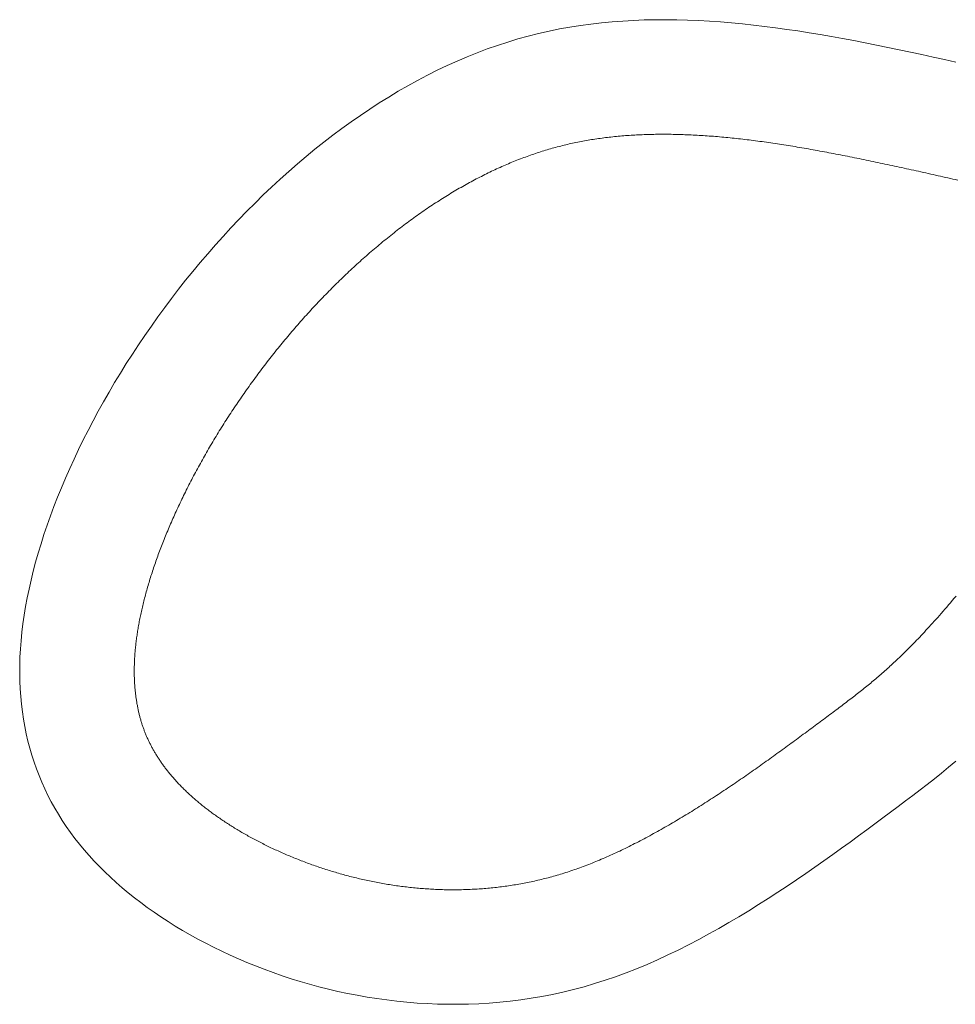
# Model space of a CAD drawing. Units: inches. Extents: x 64 to 1167, y 117 to 939.
# Tile 8 of 56: x 226.276 to 230.36, y 590.449 to 594.746. Entities that reach past the tile are written whole.
import ezdxf

# ---------------------------------------------------------------- set-up
doc = ezdxf.new("R2010")
doc.units = ezdxf.units.IN
doc.header["$MEASUREMENT"] = 0
doc.layers.add('A-FLOR-FIXT', color=8, linetype='Continuous', lineweight=18)

# ---------------------------------------------------------------- blocks, each defined once
blk = doc.blocks.new('FAUCET')
for points in [[(4.0816, 3.6354, 0), (4.1129, 3.6621, 0), (4.144, 3.6879, 0), (4.175, 3.713, 0), (4.2059, 3.7375, 0), (4.2371, 3.7616, 0), (4.2685, 3.7856, 0), (4.3004, 3.8096, 0), (4.3329, 3.8338, 0), (4.366, 3.8585, 0), (4.3999, 3.8837, 0), (4.4345, 3.9094, 0), (4.4699, 3.9356, 0), (4.506, 3.9621, 0), (4.5427, 3.989, 0), (4.5802, 4.0161, 0), (4.6182, 4.0434, 0), (4.6569, 4.0709, 0), (4.6961, 4.0984, 0), (4.7359, 4.126, 0), (4.7762, 4.1535, 0), (4.817, 4.181, 0), (4.8584, 4.2082, 0), (4.9002, 4.2353, 0), (4.9424, 4.2621, 0), (4.985, 4.2886, 0), (5.0281, 4.3147, 0), (5.0715, 4.3404, 0), (5.1152, 4.3655, 0), (5.1593, 4.3901, 0), (5.2036, 4.4141, 0), (5.2483, 4.4374, 0), (5.2931, 4.46, 0), (5.3382, 4.4817, 0), (5.3835, 4.5026, 0), (5.429, 4.5226, 0), (5.4746, 4.5416, 0), (5.5203, 4.5596, 0), (5.5662, 4.5765, 0), (5.6121, 4.5923, 0), (5.6581, 4.6068, 0), (5.7041, 4.6202, 0), (5.7502, 4.6325, 0), (5.7962, 4.6436, 0), (5.8423, 4.6537, 0), (5.8883, 4.6626, 0), (5.9343, 4.6705, 0), (5.9802, 4.6773, 0), (6.0261, 4.6831, 0), (6.0718, 4.6878, 0), (6.1175, 4.6916, 0), (6.163, 4.6944, 0), (6.2084, 4.6962, 0), (6.2536, 4.697, 0), (6.2986, 4.697, 0), (6.3435, 4.696, 0), (6.3882, 4.6942, 0), (6.4326, 4.6915, 0), (6.4768, 4.6879, 0), (6.5207, 4.6835, 0), (6.5644, 4.6782, 0), (6.6078, 4.6722, 0), (6.6509, 4.6654, 0), (6.6936, 4.6578, 0), (6.736, 4.6495, 0), (6.7781, 4.6405, 0), (6.8198, 4.6308, 0), (6.8611, 4.6203, 0), (6.902, 4.6092, 0), (6.9425, 4.5975, 0), (6.9825, 4.5851, 0), (7.0221, 4.5721, 0), (7.0612, 4.5585, 0), (7.0999, 4.5443, 0), (7.138, 4.5295, 0), (7.1756, 4.5143, 0), (7.2127, 4.4985, 0), (7.2492, 4.4821, 0), (7.2852, 4.4653, 0), (7.3206, 4.4481, 0), (7.3553, 4.4303, 0), (7.3895, 4.4122, 0), (7.423, 4.3936, 0), (7.4559, 4.3746, 0), (7.4881, 4.3553, 0), (7.5196, 4.3356, 0), (7.5504, 4.3155, 0), (7.5806, 4.2951, 0), (7.61, 4.2744, 0), (7.6387, 4.2533, 0), (7.6666, 4.2319, 0), (7.6939, 4.2101, 0), (7.7205, 4.188, 0), (7.7463, 4.1655, 0), (7.7714, 4.1426, 0), (7.7957, 4.1195, 0), (7.8193, 4.0959, 0), (7.8422, 4.072, 0), (7.8643, 4.0478, 0), (7.8857, 4.0231, 0), (7.9064, 3.9982, 0), (7.9262, 3.9728, 0), (7.9454, 3.9471, 0), (7.9637, 3.921, 0), (7.9813, 3.8946, 0), (7.9981, 3.8678, 0), (8.0142, 3.8406, 0), (8.0294, 3.8131, 0), (8.0439, 3.7852, 0), (8.0576, 3.7569, 0), (8.0705, 3.7282, 0), (8.0827, 3.6991, 0), (8.094, 3.6697, 0), (8.1045, 3.6399, 0), (8.1142, 3.6097, 0), (8.1231, 3.5791, 0), (8.1312, 3.5482, 0), (8.1385, 3.5168, 0), (8.145, 3.4851, 0), (8.1507, 3.453, 0), (8.1555, 3.4204, 0), (8.1595, 3.3875, 0), (8.1626, 3.3542, 0), (8.165, 3.3205, 0), (8.1665, 3.2864, 0), (8.1671, 3.252, 0), (8.1669, 3.2171, 0), (8.1659, 3.1818, 0), (8.164, 3.1461, 0), (8.1612, 3.11, 0), (8.1576, 3.0735, 0), (8.1531, 3.0366, 0), (8.1477, 2.9992, 0), (8.1415, 2.9615, 0), (8.1344, 2.9234, 0), (8.1264, 2.8849, 0), (8.1176, 2.846, 0), (8.108, 2.8068, 0), (8.0975, 2.7673, 0), (8.0862, 2.7275, 0), (8.074, 2.6874, 0), (8.0611, 2.647, 0), (8.0474, 2.6065, 0), (8.0329, 2.5657, 0), (8.0176, 2.5247, 0), (8.0016, 2.4835, 0), (7.9848, 2.4422, 0), (7.9672, 2.4008, 0), (7.9489, 2.3592, 0), (7.9299, 2.3176, 0), (7.9102, 2.2759, 0), (7.8898, 2.2341, 0), (7.8686, 2.1924, 0), (7.8468, 2.1506, 0), (7.8243, 2.1088, 0), (7.8011, 2.0671, 0), (7.7772, 2.0254, 0), (7.7527, 1.9838, 0), (7.7276, 1.9423, 0), (7.7018, 1.9009, 0), (7.6754, 1.8597, 0), (7.6484, 1.8186, 0), (7.6207, 1.7777, 0), (7.5925, 1.737, 0), (7.5637, 1.6965, 0), (7.5343, 1.6563, 0), (7.5043, 1.6163, 0), (7.4738, 1.5766, 0), (7.4428, 1.5372, 0), (7.4112, 1.4981, 0), (7.379, 1.4594, 0), (7.3464, 1.4211, 0), (7.3132, 1.3831, 0), (7.2795, 1.3456, 0), (7.2453, 1.3085, 0), (7.2107, 1.2718, 0), (7.1755, 1.2356, 0), (7.1399, 1.1999, 0), (7.1039, 1.1647, 0), (7.0674, 1.13, 0), (7.0305, 1.0959, 0), (6.9931, 1.0624, 0), (6.9553, 1.0294, 0), (6.9171, 0.9971, 0), (6.8785, 0.9654, 0), (6.8396, 0.9344, 0), (6.8002, 0.904, 0), (6.7605, 0.8744, 0), (6.7204, 0.8455, 0), (6.6799, 0.8173, 0), (6.6391, 0.7898, 0), (6.598, 0.7632, 0), (6.5566, 0.7373, 0), (6.5148, 0.7123, 0), (6.4727, 0.6881, 0), (6.4304, 0.6648, 0), (6.3877, 0.6424, 0), (6.3448, 0.6208, 0), (6.3016, 0.6002, 0), (6.2581, 0.5806, 0), (6.2144, 0.5619, 0), (6.1705, 0.5442, 0), (6.1263, 0.5275, 0), (6.0819, 0.5119, 0), (6.0373, 0.4973, 0), (5.9925, 0.4837, 0), (5.9475, 0.4713, 0), (5.9023, 0.4599, 0), (5.8569, 0.4497, 0), (5.8114, 0.4404, 0), (5.7657, 0.4322, 0), (5.7198, 0.425, 0), (5.6737, 0.4187, 0), (5.6275, 0.4134, 0), (5.5811, 0.409, 0), (5.5345, 0.4055, 0), (5.4878, 0.4029, 0), (5.441, 0.401, 0), (5.394, 0.4, 0), (5.3468, 0.3998, 0), (5.2995, 0.4004, 0), (5.2521, 0.4017, 0), (5.2045, 0.4036, 0), (5.1568, 0.4063, 0), (5.109, 0.4096, 0), (5.0611, 0.4136, 0), (5.013, 0.4182, 0), (4.9648, 0.4233, 0), (4.9165, 0.429, 0), (4.8681, 0.4352, 0), (4.8196, 0.4419, 0), (4.771, 0.4491, 0), (4.7222, 0.4568, 0), (4.6734, 0.4648, 0), (4.6245, 0.4733, 0), (4.5755, 0.4822, 0), (4.5264, 0.4913, 0), (4.4772, 0.5008, 0), (4.428, 0.5106, 0), (4.3786, 0.5207, 0), (4.3292, 0.531, 0), (4.2798, 0.5415, 0), (4.2302, 0.5522, 0), (4.1806, 0.5631, 0), (4.131, 0.5741, 0), (4.0812, 0.5853, 0)], [(4.0798, 2.9151, 0), (4.0883, 2.9251, 0), (4.0967, 2.935, 0), (4.1049, 2.9447, 0), (4.1131, 2.9542, 0), (4.1212, 2.9636, 0), (4.1292, 2.9729, 0), (4.1371, 2.9819, 0), (4.145, 2.9909, 0), (4.1527, 2.9996, 0), (4.1603, 3.0083, 0), (4.1679, 3.0168, 0), (4.1754, 3.0251, 0), (4.1828, 3.0333, 0), (4.1901, 3.0414, 0), (4.1973, 3.0493, 0), (4.2045, 3.0572, 0), (4.2116, 3.0648, 0), (4.2186, 3.0724, 0), (4.2256, 3.0798, 0), (4.2324, 3.0871, 0), (4.2392, 3.0943, 0), (4.246, 3.1013, 0), (4.2526, 3.1083, 0), (4.2592, 3.1151, 0), (4.2658, 3.1219, 0), (4.2722, 3.1285, 0), (4.2786, 3.135, 0), (4.285, 3.1414, 0), (4.2913, 3.1477, 0), (4.2975, 3.1539, 0), (4.3037, 3.16, 0), (4.3098, 3.166, 0), (4.3159, 3.1719, 0), (4.3219, 3.1777, 0), (4.3279, 3.1835, 0), (4.3338, 3.1891, 0), (4.3397, 3.1947, 0), (4.3456, 3.2002, 0), (4.3514, 3.2057, 0), (4.3572, 3.211, 0), (4.3629, 3.2164, 0), (4.3687, 3.2216, 0), (4.3744, 3.2268, 0), (4.3801, 3.2319, 0), (4.3857, 3.237, 0), (4.3914, 3.242, 0), (4.397, 3.247, 0), (4.4026, 3.252, 0), (4.4082, 3.2569, 0), (4.4138, 3.2617, 0), (4.4194, 3.2665, 0), (4.425, 3.2713, 0), (4.4306, 3.2761, 0), (4.4362, 3.2808, 0), (4.4418, 3.2855, 0), (4.4474, 3.2902, 0), (4.453, 3.2948, 0), (4.4587, 3.2995, 0), (4.4643, 3.3041, 0), (4.47, 3.3087, 0), (4.4756, 3.3133, 0), (4.4813, 3.3179, 0), (4.4871, 3.3224, 0), (4.4928, 3.327, 0), (4.4986, 3.3316, 0), (4.5044, 3.3362, 0), (4.5103, 3.3408, 0), (4.5161, 3.3454, 0), (4.5221, 3.35, 0), (4.528, 3.3546, 0), (4.534, 3.3592, 0), (4.5401, 3.3639, 0), (4.5462, 3.3685, 0), (4.5523, 3.3732, 0), (4.5585, 3.378, 0), (4.5648, 3.3827, 0), (4.5711, 3.3875, 0), (4.5775, 3.3923, 0), (4.5839, 3.3972, 0), (4.5905, 3.4021, 0), (4.597, 3.407, 0), (4.6037, 3.412, 0), (4.6104, 3.417, 0), (4.6172, 3.4221, 0), (4.624, 3.4272, 0), (4.6309, 3.4324, 0), (4.6379, 3.4376, 0), (4.6448, 3.4428, 0), (4.6519, 3.448, 0), (4.659, 3.4533, 0), (4.6661, 3.4586, 0), (4.6733, 3.464, 0), (4.6805, 3.4694, 0), (4.6877, 3.4748, 0), (4.695, 3.4802, 0), (4.7024, 3.4856, 0), (4.7097, 3.4911, 0), (4.7171, 3.4966, 0), (4.7246, 3.5021, 0), (4.732, 3.5076, 0), (4.7395, 3.5132, 0), (4.747, 3.5187, 0), (4.7546, 3.5243, 0), (4.7621, 3.5299, 0), (4.7697, 3.5355, 0), (4.7773, 3.541, 0), (4.7849, 3.5466, 0), (4.7926, 3.5523, 0), (4.8002, 3.5579, 0), (4.8079, 3.5635, 0), (4.8156, 3.5691, 0), (4.8232, 3.5747, 0), (4.8309, 3.5803, 0), (4.8386, 3.5859, 0), (4.8464, 3.5915, 0), (4.8541, 3.5972, 0), (4.8619, 3.6028, 0), (4.8696, 3.6084, 0), (4.8774, 3.614, 0), (4.8852, 3.6196, 0), (4.8931, 3.6253, 0), (4.9009, 3.6309, 0), (4.9088, 3.6365, 0), (4.9167, 3.6421, 0), (4.9246, 3.6478, 0), (4.9325, 3.6534, 0), (4.9404, 3.659, 0), (4.9484, 3.6646, 0), (4.9563, 3.6702, 0), (4.9643, 3.6758, 0), (4.9723, 3.6814, 0), (4.9803, 3.687, 0), (4.9883, 3.6926, 0), (4.9964, 3.6982, 0), (5.0044, 3.7038, 0), (5.0125, 3.7094, 0), (5.0206, 3.7149, 0), (5.0286, 3.7205, 0), (5.0367, 3.726, 0), (5.0449, 3.7316, 0), (5.053, 3.7371, 0), (5.0611, 3.7426, 0), (5.0693, 3.7481, 0), (5.0774, 3.7536, 0), (5.0856, 3.7591, 0), (5.0938, 3.7645, 0), (5.102, 3.77, 0), (5.1102, 3.7754, 0), (5.1184, 3.7808, 0), (5.1266, 3.7862, 0), (5.1349, 3.7916, 0), (5.1431, 3.797, 0), (5.1514, 3.8023, 0), (5.1596, 3.8077, 0), (5.1679, 3.813, 0), (5.1762, 3.8183, 0), (5.1844, 3.8235, 0), (5.1927, 3.8288, 0), (5.201, 3.834, 0), (5.2093, 3.8393, 0), (5.2176, 3.8444, 0), (5.2259, 3.8496, 0), (5.2342, 3.8548, 0), (5.2425, 3.8599, 0), (5.2509, 3.865, 0), (5.2592, 3.8701, 0), (5.2675, 3.8751, 0), (5.2758, 3.8801, 0), (5.2841, 3.8851, 0), (5.2925, 3.8901, 0), (5.3008, 3.8951, 0), (5.3091, 3.9, 0), (5.3174, 3.9049, 0), (5.3258, 3.9097, 0), (5.3341, 3.9146, 0), (5.3424, 3.9194, 0), (5.3507, 3.9241, 0), (5.359, 3.9289, 0), (5.3673, 3.9336, 0), (5.3757, 3.9382, 0), (5.384, 3.9429, 0), (5.3923, 3.9475, 0), (5.4005, 3.9521, 0), (5.4088, 3.9566, 0), (5.4171, 3.9611, 0), (5.4254, 3.9656, 0), (5.4337, 3.97, 0), (5.4419, 3.9744, 0), (5.4502, 3.9788, 0), (5.4584, 3.9831, 0), (5.4667, 3.9874, 0), (5.4749, 3.9916, 0), (5.4831, 3.9959, 0), (5.4913, 4, 0), (5.4995, 4.0042, 0), (5.5077, 4.0082, 0), (5.5159, 4.0123, 0), (5.5241, 4.0163, 0), (5.5322, 4.0203, 0), (5.5403, 4.0242, 0), (5.5485, 4.028, 0), (5.5566, 4.0319, 0), (5.5647, 4.0357, 0), (5.5728, 4.0394, 0), (5.5808, 4.0431, 0), (5.5889, 4.0467, 0), (5.5969, 4.0503, 0), (5.6049, 4.0539, 0), (5.6129, 4.0574, 0), (5.6209, 4.0608, 0), (5.6288, 4.0642, 0), (5.6367, 4.0676, 0), (5.6446, 4.0708, 0), (5.6525, 4.0741, 0), (5.6604, 4.0773, 0), (5.6682, 4.0804, 0), (5.676, 4.0835, 0), (5.6838, 4.0866, 0), (5.6916, 4.0896, 0), (5.6994, 4.0926, 0), (5.7072, 4.0955, 0), (5.7149, 4.0983, 0), (5.7226, 4.1012, 0), (5.7304, 4.1039, 0), (5.7381, 4.1067, 0), (5.7457, 4.1093, 0), (5.7534, 4.112, 0), (5.7611, 4.1146, 0), (5.7687, 4.1171, 0), (5.7764, 4.1196, 0), (5.784, 4.1221, 0), (5.7916, 4.1245, 0), (5.7992, 4.1269, 0), (5.8069, 4.1292, 0), (5.8144, 4.1315, 0), (5.822, 4.1337, 0), (5.8296, 4.1359, 0), (5.8372, 4.1381, 0), (5.8448, 4.1402, 0), (5.8523, 4.1422, 0), (5.8599, 4.1443, 0), (5.8674, 4.1462, 0), (5.875, 4.1482, 0), (5.8825, 4.1501, 0), (5.89, 4.1519, 0), (5.8976, 4.1538, 0), (5.9051, 4.1555, 0), (5.9126, 4.1573, 0), (5.9202, 4.159, 0), (5.9277, 4.1606, 0), (5.9352, 4.1623, 0), (5.9428, 4.1638, 0), (5.9503, 4.1654, 0), (5.9578, 4.1669, 0), (5.9654, 4.1683, 0), (5.9729, 4.1698, 0), (5.9804, 4.1712, 0), (5.988, 4.1725, 0), (5.9955, 4.1738, 0), (6.0031, 4.1751, 0), (6.0106, 4.1763, 0), (6.0182, 4.1775, 0), (6.0257, 4.1787, 0), (6.0333, 4.1798, 0), (6.0409, 4.1809, 0), (6.0485, 4.182, 0), (6.056, 4.183, 0), (6.0636, 4.184, 0), (6.0712, 4.1849, 0), (6.0788, 4.1858, 0), (6.0864, 4.1867, 0), (6.094, 4.1875, 0), (6.1016, 4.1883, 0), (6.1092, 4.1891, 0), (6.1168, 4.1898, 0), (6.1244, 4.1905, 0), (6.132, 4.1912, 0), (6.1396, 4.1918, 0), (6.1472, 4.1924, 0), (6.1548, 4.193, 0), (6.1624, 4.1935, 0), (6.17, 4.194, 0), (6.1776, 4.1944, 0), (6.1852, 4.1948, 0), (6.1928, 4.1952, 0), (6.2004, 4.1956, 0), (6.208, 4.1959, 0), (6.2155, 4.1961, 0), (6.2231, 4.1964, 0), (6.2307, 4.1966, 0), (6.2383, 4.1968, 0), (6.2459, 4.1969, 0), (6.2534, 4.197, 0), (6.261, 4.1971, 0), (6.2686, 4.1971, 0), (6.2761, 4.1971, 0), (6.2837, 4.1971, 0), (6.2913, 4.197, 0), (6.2988, 4.1969, 0), (6.3064, 4.1968, 0), (6.3139, 4.1967, 0), (6.3215, 4.1965, 0), (6.329, 4.1962, 0), (6.3365, 4.196, 0), (6.3441, 4.1957, 0), (6.3516, 4.1954, 0), (6.3591, 4.195, 0), (6.3666, 4.1946, 0), (6.3741, 4.1942, 0), (6.3817, 4.1937, 0), (6.3892, 4.1933, 0), (6.3967, 4.1927, 0), (6.4042, 4.1922, 0), (6.4116, 4.1916, 0), (6.4191, 4.191, 0), (6.4266, 4.1904, 0), (6.4341, 4.1897, 0), (6.4415, 4.189, 0), (6.449, 4.1883, 0), (6.4564, 4.1875, 0), (6.4639, 4.1867, 0), (6.4713, 4.1859, 0), (6.4788, 4.185, 0), (6.4862, 4.1841, 0), (6.4936, 4.1832, 0), (6.501, 4.1823, 0), (6.5084, 4.1813, 0), (6.5158, 4.1803, 0), (6.5232, 4.1793, 0), (6.5306, 4.1782, 0), (6.5379, 4.1771, 0), (6.5453, 4.176, 0), (6.5527, 4.1748, 0), (6.56, 4.1736, 0), (6.5673, 4.1724, 0), (6.5747, 4.1712, 0), (6.582, 4.1699, 0), (6.5893, 4.1686, 0), (6.5966, 4.1673, 0), (6.6039, 4.1659, 0), (6.6112, 4.1645, 0), (6.6185, 4.1631, 0), (6.6257, 4.1616, 0), (6.633, 4.1602, 0), (6.6402, 4.1587, 0), (6.6474, 4.1571, 0), (6.6546, 4.1556, 0), (6.6618, 4.154, 0), (6.669, 4.1524, 0), (6.6762, 4.1507, 0), (6.6834, 4.1491, 0), (6.6905, 4.1474, 0), (6.6977, 4.1457, 0), (6.7048, 4.1439, 0), (6.7119, 4.1421, 0), (6.719, 4.1403, 0), (6.7261, 4.1385, 0), (6.7332, 4.1367, 0), (6.7403, 4.1348, 0), (6.7473, 4.1329, 0), (6.7543, 4.131, 0), (6.7613, 4.129, 0), (6.7683, 4.1271, 0), (6.7753, 4.1251, 0), (6.7823, 4.123, 0), (6.7893, 4.121, 0), (6.7962, 4.1189, 0), (6.8031, 4.1168, 0), (6.81, 4.1147, 0), (6.8169, 4.1126, 0), (6.8238, 4.1104, 0), (6.8307, 4.1082, 0), (6.8375, 4.106, 0), (6.8443, 4.1038, 0), (6.8511, 4.1016, 0), (6.8579, 4.0993, 0), (6.8647, 4.097, 0), (6.8714, 4.0947, 0), (6.8782, 4.0924, 0), (6.8849, 4.09, 0), (6.8916, 4.0876, 0), (6.8982, 4.0852, 0), (6.9049, 4.0828, 0), (6.9115, 4.0804, 0), (6.9181, 4.0779, 0), (6.9247, 4.0754, 0), (6.9313, 4.0729, 0), (6.9379, 4.0704, 0), (6.9444, 4.0679, 0), (6.9509, 4.0653, 0), (6.9574, 4.0628, 0), (6.9639, 4.0602, 0), (6.9703, 4.0576, 0), (6.9767, 4.0549, 0), (6.9831, 4.0523, 0), (6.9895, 4.0496, 0), (6.9959, 4.047, 0), (7.0022, 4.0443, 0), (7.0085, 4.0415, 0), (7.0148, 4.0388, 0), (7.0211, 4.0361, 0), (7.0273, 4.0333, 0), (7.0335, 4.0305, 0), (7.0397, 4.0277, 0), (7.0459, 4.0249, 0), (7.052, 4.0221, 0), (7.0582, 4.0192, 0), (7.0642, 4.0164, 0), (7.0703, 4.0135, 0), (7.0764, 4.0106, 0), (7.0824, 4.0077, 0), (7.0884, 4.0048, 0), (7.0943, 4.0018, 0), (7.1003, 3.9989, 0), (7.1062, 3.9959, 0), (7.1121, 3.9929, 0), (7.1179, 3.99, 0), (7.1238, 3.987, 0), (7.1296, 3.9839, 0), (7.1353, 3.9809, 0), (7.1411, 3.9779, 0), (7.1468, 3.9748, 0), (7.1525, 3.9717, 0), (7.1582, 3.9687, 0), (7.1638, 3.9656, 0), (7.1694, 3.9625, 0), (7.175, 3.9593, 0), (7.1805, 3.9562, 0), (7.186, 3.9531, 0), (7.1915, 3.9499, 0), (7.197, 3.9468, 0), (7.2024, 3.9436, 0), (7.2078, 3.9404, 0), (7.2131, 3.9372, 0), (7.2185, 3.934, 0), (7.2238, 3.9308, 0), (7.229, 3.9276, 0), (7.2343, 3.9244, 0), (7.2395, 3.9211, 0), (7.2447, 3.9179, 0), (7.2498, 3.9146, 0), (7.2549, 3.9114, 0), (7.26, 3.9081, 0), (7.265, 3.9048, 0), (7.27, 3.9015, 0), (7.2749, 3.8983, 0), (7.2798, 3.895, 0), (7.2847, 3.8917, 0), (7.2895, 3.8884, 0), (7.2943, 3.8851, 0), (7.2991, 3.8819, 0), (7.3038, 3.8786, 0), (7.3085, 3.8753, 0), (7.3131, 3.872, 0), (7.3177, 3.8687, 0), (7.3223, 3.8654, 0), (7.3268, 3.8621, 0), (7.3313, 3.8588, 0), (7.3357, 3.8555, 0), (7.3401, 3.8522, 0), (7.3445, 3.8489, 0), (7.3488, 3.8456, 0), (7.3531, 3.8423, 0), (7.3574, 3.839, 0), (7.3616, 3.8357, 0), (7.3658, 3.8324, 0), (7.37, 3.8291, 0), (7.3741, 3.8258, 0), (7.3782, 3.8224, 0), (7.3822, 3.8191, 0), (7.3862, 3.8158, 0), (7.3902, 3.8125, 0), (7.3941, 3.8092, 0), (7.398, 3.8059, 0), (7.4019, 3.8025, 0), (7.4057, 3.7992, 0), (7.4095, 3.7959, 0), (7.4133, 3.7926, 0), (7.417, 3.7892, 0), (7.4207, 3.7859, 0), (7.4243, 3.7826, 0), (7.4279, 3.7793, 0), (7.4315, 3.7759, 0), (7.4351, 3.7726, 0), (7.4386, 3.7693, 0), (7.4421, 3.7659, 0), (7.4455, 3.7626, 0), (7.4489, 3.7593, 0), (7.4523, 3.7559, 0), (7.4557, 3.7526, 0), (7.459, 3.7493, 0), (7.4623, 3.7459, 0), (7.4655, 3.7426, 0), (7.4687, 3.7393, 0), (7.4719, 3.7359, 0), (7.4751, 3.7326, 0), (7.4782, 3.7293, 0), (7.4813, 3.7259, 0), (7.4843, 3.7226, 0), (7.4874, 3.7193, 0), (7.4903, 3.7159, 0), (7.4933, 3.7126, 0), (7.4962, 3.7093, 0), (7.4991, 3.7059, 0), (7.502, 3.7026, 0), (7.5048, 3.6992, 0), (7.5076, 3.6959, 0), (7.5104, 3.6926, 0), (7.5132, 3.6892, 0), (7.5159, 3.6859, 0), (7.5185, 3.6826, 0), (7.5212, 3.6792, 0), (7.5238, 3.6759, 0), (7.5264, 3.6726, 0), (7.529, 3.6692, 0), (7.5315, 3.6659, 0), (7.534, 3.6626, 0), (7.5365, 3.6592, 0), (7.5389, 3.6559, 0), (7.5413, 3.6526, 0), (7.5437, 3.6492, 0), (7.5461, 3.6459, 0), (7.5484, 3.6426, 0), (7.5507, 3.6392, 0), (7.553, 3.6359, 0), (7.5552, 3.6326, 0), (7.5574, 3.6293, 0), (7.5597, 3.6259, 0), (7.5618, 3.6226, 0), (7.564, 3.6193, 0), (7.5661, 3.6159, 0), (7.5682, 3.6126, 0), (7.5703, 3.6092, 0), (7.5724, 3.6059, 0), (7.5744, 3.6026, 0), (7.5764, 3.5992, 0), (7.5784, 3.5959, 0), (7.5803, 3.5925, 0), (7.5823, 3.5891, 0), (7.5842, 3.5858, 0), (7.5861, 3.5824, 0), (7.5879, 3.579, 0), (7.5898, 3.5757, 0), (7.5916, 3.5723, 0), (7.5934, 3.5689, 0), (7.5952, 3.5655, 0), (7.5969, 3.5621, 0), (7.5987, 3.5587, 0), (7.6004, 3.5553, 0), (7.602, 3.5518, 0), (7.6037, 3.5484, 0), (7.6053, 3.545, 0), (7.6069, 3.5415, 0), (7.6085, 3.538, 0), (7.6101, 3.5346, 0), (7.6116, 3.5311, 0), (7.6132, 3.5276, 0), (7.6147, 3.5241, 0), (7.6161, 3.5206, 0), (7.6176, 3.5171, 0), (7.619, 3.5136, 0), (7.6204, 3.51, 0), (7.6218, 3.5065, 0), (7.6232, 3.5029, 0), (7.6245, 3.4994, 0), (7.6259, 3.4958, 0), (7.6272, 3.4922, 0), (7.6284, 3.4886, 0), (7.6297, 3.4849, 0), (7.6309, 3.4813, 0), (7.6322, 3.4777, 0), (7.6333, 3.474, 0), (7.6345, 3.4703, 0), (7.6357, 3.4666, 0), (7.6368, 3.4629, 0), (7.6379, 3.4592, 0), (7.639, 3.4555, 0), (7.6401, 3.4517, 0), (7.6411, 3.4479, 0), (7.6421, 3.4441, 0), (7.6432, 3.4403, 0), (7.6441, 3.4365, 0), (7.6451, 3.4327, 0), (7.646, 3.4288, 0), (7.647, 3.4249, 0), (7.6479, 3.4211, 0), (7.6488, 3.4171, 0), (7.6496, 3.4132, 0), (7.6505, 3.4093, 0), (7.6513, 3.4053, 0), (7.6521, 3.4013, 0), (7.6529, 3.3973, 0), (7.6536, 3.3933, 0), (7.6544, 3.3892, 0), (7.6551, 3.3852, 0), (7.6558, 3.3811, 0), (7.6565, 3.377, 0), (7.6572, 3.3728, 0), (7.6578, 3.3687, 0), (7.6584, 3.3645, 0), (7.6591, 3.3603, 0), (7.6596, 3.3561, 0), (7.6602, 3.3518, 0), (7.6608, 3.3475, 0), (7.6613, 3.3432, 0), (7.6618, 3.3389, 0), (7.6623, 3.3346, 0), (7.6628, 3.3302, 0), (7.6632, 3.3258, 0), (7.6636, 3.3213, 0), (7.664, 3.3169, 0), (7.6644, 3.3124, 0), (7.6647, 3.3079, 0), (7.6651, 3.3033, 0), (7.6654, 3.2988, 0), (7.6657, 3.2941, 0), (7.6659, 3.2895, 0), (7.6661, 3.2849, 0), (7.6663, 3.2802, 0), (7.6665, 3.2755, 0), (7.6667, 3.2707, 0), (7.6668, 3.2659, 0), (7.6669, 3.2611, 0), (7.667, 3.2563, 0), (7.6671, 3.2514, 0), (7.6671, 3.2466, 0), (7.6671, 3.2416, 0), (7.6671, 3.2367, 0), (7.667, 3.2317, 0), (7.6669, 3.2267, 0), (7.6668, 3.2217, 0), (7.6667, 3.2166, 0), (7.6666, 3.2115, 0), (7.6664, 3.2064, 0), (7.6662, 3.2012, 0), (7.6659, 3.1961, 0), (7.6657, 3.1908, 0), (7.6654, 3.1856, 0), (7.665, 3.1803, 0), (7.6647, 3.175, 0), (7.6643, 3.1697, 0), (7.6639, 3.1643, 0), (7.6635, 3.1589, 0), (7.663, 3.1535, 0), (7.6625, 3.148, 0), (7.662, 3.1426, 0), (7.6614, 3.137, 0), (7.6608, 3.1315, 0), (7.6602, 3.1259, 0), (7.6596, 3.1203, 0), (7.6589, 3.1147, 0), (7.6582, 3.109, 0), (7.6574, 3.1033, 0), (7.6567, 3.0975, 0), (7.6559, 3.0918, 0), (7.655, 3.086, 0), (7.6542, 3.0801, 0), (7.6533, 3.0743, 0), (7.6524, 3.0684, 0), (7.6514, 3.0625, 0), (7.6504, 3.0565, 0), (7.6494, 3.0505, 0), (7.6483, 3.0445, 0), (7.6472, 3.0384, 0), (7.6461, 3.0324, 0), (7.645, 3.0262, 0), (7.6438, 3.0201, 0), (7.6425, 3.0139, 0), (7.6413, 3.0077, 0), (7.64, 3.0014, 0), (7.6387, 2.9951, 0), (7.6373, 2.9888, 0), (7.6359, 2.9825, 0), (7.6345, 2.9761, 0), (7.633, 2.9697, 0), (7.6315, 2.9632, 0), (7.63, 2.9567, 0), (7.6284, 2.9502, 0), (7.6268, 2.9437, 0), (7.6252, 2.9371, 0), (7.6235, 2.9305, 0), (7.6218, 2.9238, 0), (7.62, 2.9171, 0), (7.6182, 2.9104, 0), (7.6164, 2.9037, 0), (7.6146, 2.8969, 0), (7.6127, 2.8901, 0), (7.6107, 2.8832, 0), (7.6088, 2.8764, 0), (7.6067, 2.8695, 0), (7.6047, 2.8626, 0), (7.6026, 2.8556, 0), (7.6005, 2.8487, 0), (7.5984, 2.8417, 0), (7.5962, 2.8347, 0), (7.594, 2.8277, 0), (7.5917, 2.8206, 0), (7.5894, 2.8135, 0), (7.5871, 2.8064, 0), (7.5848, 2.7993, 0), (7.5824, 2.7921, 0), (7.58, 2.785, 0), (7.5775, 2.7778, 0), (7.575, 2.7706, 0), (7.5725, 2.7634, 0), (7.5699, 2.7561, 0), (7.5673, 2.7488, 0), (7.5647, 2.7415, 0), (7.562, 2.7342, 0), (7.5593, 2.7269, 0), (7.5566, 2.7196, 0), (7.5538, 2.7122, 0), (7.551, 2.7048, 0), (7.5482, 2.6974, 0), (7.5453, 2.69, 0), (7.5424, 2.6826, 0), (7.5395, 2.6751, 0), (7.5365, 2.6677, 0), (7.5335, 2.6602, 0), (7.5305, 2.6527, 0), (7.5274, 2.6452, 0), (7.5243, 2.6376, 0), (7.5212, 2.6301, 0), (7.518, 2.6225, 0), (7.5148, 2.615, 0), (7.5116, 2.6074, 0), (7.5083, 2.5998, 0), (7.505, 2.5922, 0), (7.5017, 2.5846, 0), (7.4984, 2.5769, 0), (7.495, 2.5693, 0), (7.4915, 2.5616, 0), (7.4881, 2.554, 0), (7.4846, 2.5463, 0), (7.4811, 2.5386, 0), (7.4775, 2.5309, 0), (7.4739, 2.5232, 0), (7.4703, 2.5155, 0), (7.4667, 2.5077, 0), (7.463, 2.5, 0), (7.4593, 2.4923, 0), (7.4555, 2.4845, 0), (7.4518, 2.4767, 0), (7.448, 2.469, 0), (7.4441, 2.4612, 0), (7.4403, 2.4534, 0), (7.4364, 2.4456, 0), (7.4324, 2.4378, 0), (7.4285, 2.43, 0), (7.4245, 2.4222, 0), (7.4205, 2.4144, 0), (7.4164, 2.4066, 0), (7.4123, 2.3987, 0), (7.4082, 2.3909, 0), (7.4041, 2.3831, 0), (7.3999, 2.3753, 0), (7.3957, 2.3674, 0), (7.3915, 2.3596, 0), (7.3872, 2.3517, 0), (7.3829, 2.3439, 0), (7.3786, 2.336, 0), (7.3742, 2.3282, 0), (7.3699, 2.3203, 0), (7.3654, 2.3125, 0), (7.361, 2.3046, 0), (7.3565, 2.2968, 0), (7.352, 2.2889, 0), (7.3475, 2.2811, 0), (7.3429, 2.2732, 0), (7.3383, 2.2653, 0), (7.3337, 2.2575, 0), (7.3291, 2.2496, 0), (7.3244, 2.2418, 0), (7.3197, 2.2339, 0), (7.315, 2.2261, 0), (7.3102, 2.2182, 0), (7.3054, 2.2104, 0), (7.3006, 2.2026, 0), (7.2958, 2.1947, 0), (7.2909, 2.1869, 0), (7.286, 2.1791, 0), (7.2811, 2.1712, 0), (7.2762, 2.1634, 0), (7.2712, 2.1556, 0), (7.2662, 2.1478, 0), (7.2612, 2.1399, 0), (7.2561, 2.1321, 0), (7.251, 2.1243, 0), (7.2459, 2.1165, 0), (7.2408, 2.1087, 0), (7.2356, 2.1009, 0), (7.2304, 2.0932, 0), (7.2252, 2.0854, 0), (7.22, 2.0776, 0), (7.2147, 2.0699, 0), (7.2094, 2.0621, 0), (7.2041, 2.0543, 0), (7.1988, 2.0466, 0), (7.1934, 2.0389, 0), (7.188, 2.0311, 0), (7.1826, 2.0234, 0), (7.1772, 2.0157, 0), (7.1717, 2.008, 0), (7.1662, 2.0003, 0), (7.1607, 1.9926, 0), (7.1552, 1.985, 0), (7.1496, 1.9773, 0), (7.144, 1.9697, 0), (7.1384, 1.962, 0), (7.1328, 1.9544, 0), (7.1272, 1.9468, 0), (7.1215, 1.9391, 0), (7.1158, 1.9316, 0), (7.1101, 1.924, 0), (7.1043, 1.9164, 0), (7.0986, 1.9088, 0), (7.0928, 1.9013, 0), (7.087, 1.8937, 0), (7.0811, 1.8862, 0), (7.0753, 1.8787, 0), (7.0694, 1.8712, 0), (7.0635, 1.8637, 0), (7.0576, 1.8562, 0), (7.0516, 1.8488, 0), (7.0457, 1.8413, 0), (7.0397, 1.8339, 0), (7.0337, 1.8265, 0), (7.0276, 1.8191, 0), (7.0216, 1.8117, 0), (7.0155, 1.8043, 0), (7.0094, 1.797, 0), (7.0033, 1.7896, 0), (6.9972, 1.7823, 0), (6.991, 1.775, 0), (6.9849, 1.7677, 0), (6.9787, 1.7604, 0), (6.9725, 1.7532, 0), (6.9662, 1.746, 0), (6.96, 1.7387, 0), (6.9537, 1.7315, 0), (6.9474, 1.7244, 0), (6.9411, 1.7172, 0), (6.9348, 1.71, 0), (6.9284, 1.7029, 0), (6.9221, 1.6958, 0), (6.9157, 1.6887, 0), (6.9093, 1.6817, 0), (6.9029, 1.6746, 0), (6.8964, 1.6676, 0), (6.89, 1.6606, 0), (6.8835, 1.6536, 0), (6.877, 1.6466, 0), (6.8705, 1.6397, 0), (6.864, 1.6328, 0), (6.8574, 1.6259, 0), (6.8509, 1.619, 0), (6.8443, 1.6121, 0), (6.8377, 1.6053, 0), (6.8311, 1.5985, 0), (6.8244, 1.5917, 0), (6.8178, 1.5849, 0), (6.8111, 1.5782, 0), (6.8045, 1.5715, 0), (6.7978, 1.5648, 0), (6.7911, 1.5581, 0), (6.7843, 1.5515, 0), (6.7776, 1.5448, 0), (6.7708, 1.5382, 0), (6.7641, 1.5317, 0), (6.7573, 1.5251, 0), (6.7505, 1.5186, 0), (6.7437, 1.5121, 0), (6.7368, 1.5056, 0), (6.73, 1.4992, 0), (6.7231, 1.4927, 0), (6.7163, 1.4864, 0), (6.7094, 1.48, 0), (6.7025, 1.4736, 0), (6.6956, 1.4673, 0), (6.6887, 1.461, 0), (6.6817, 1.4548, 0), (6.6748, 1.4485, 0), (6.6678, 1.4423, 0), (6.6608, 1.4361, 0), (6.6539, 1.43, 0), (6.6469, 1.4238, 0), (6.6398, 1.4177, 0), (6.6328, 1.4117, 0), (6.6258, 1.4056, 0), (6.6187, 1.3996, 0), (6.6117, 1.3936, 0), (6.6046, 1.3877, 0), (6.5975, 1.3818, 0), (6.5905, 1.3759, 0), (6.5834, 1.37, 0), (6.5763, 1.3642, 0), (6.5691, 1.3584, 0), (6.562, 1.3526, 0), (6.5549, 1.3468, 0), (6.5477, 1.3411, 0), (6.5406, 1.3354, 0), (6.5334, 1.3298, 0), (6.5262, 1.3242, 0), (6.519, 1.3186, 0), (6.5118, 1.313, 0), (6.5046, 1.3075, 0), (6.4974, 1.302, 0), (6.4902, 1.2965, 0), (6.483, 1.2911, 0), (6.4757, 1.2857, 0), (6.4685, 1.2803, 0), (6.4612, 1.275, 0), (6.454, 1.2697, 0), (6.4467, 1.2645, 0), (6.4394, 1.2592, 0), (6.4322, 1.254, 0), (6.4249, 1.2489, 0), (6.4176, 1.2438, 0), (6.4103, 1.2387, 0), (6.403, 1.2336, 0), (6.3956, 1.2286, 0), (6.3883, 1.2236, 0), (6.381, 1.2187, 0), (6.3737, 1.2137, 0), (6.3663, 1.2089, 0), (6.359, 1.204, 0), (6.3517, 1.1992, 0), (6.3443, 1.1944, 0), (6.3369, 1.1897, 0), (6.3296, 1.185, 0), (6.3222, 1.1804, 0), (6.3149, 1.1757, 0), (6.3075, 1.1711, 0), (6.3001, 1.1666, 0), (6.2927, 1.1621, 0), (6.2854, 1.1576, 0), (6.278, 1.1532, 0), (6.2706, 1.1488, 0), (6.2632, 1.1444, 0), (6.2558, 1.1401, 0), (6.2484, 1.1358, 0), (6.241, 1.1315, 0), (6.2336, 1.1273, 0), (6.2262, 1.1232, 0), (6.2188, 1.119, 0), (6.2114, 1.1149, 0), (6.204, 1.1109, 0), (6.1966, 1.1068, 0), (6.1892, 1.1029, 0), (6.1818, 1.0989, 0), (6.1744, 1.095, 0), (6.167, 1.0911, 0), (6.1595, 1.0873, 0), (6.1521, 1.0835, 0), (6.1447, 1.0798, 0), (6.1373, 1.0761, 0), (6.1299, 1.0724, 0), (6.1225, 1.0688, 0), (6.1151, 1.0652, 0), (6.1077, 1.0616, 0), (6.1003, 1.0581, 0), (6.0929, 1.0546, 0), (6.0855, 1.0512, 0), (6.0781, 1.0478, 0), (6.0707, 1.0445, 0), (6.0633, 1.0411, 0), (6.0559, 1.0379, 0), (6.0485, 1.0346, 0), (6.0411, 1.0314, 0), (6.0337, 1.0283, 0), (6.0263, 1.0252, 0), (6.0189, 1.0221, 0), (6.0115, 1.0191, 0), (6.0042, 1.0161, 0), (5.9968, 1.0132, 0), (5.9894, 1.0103, 0), (5.982, 1.0074, 0), (5.9747, 1.0046, 0), (5.9673, 1.0018, 0), (5.96, 0.9991, 0), (5.9526, 0.9964, 0), (5.9453, 0.9937, 0), (5.9379, 0.9911, 0), (5.9306, 0.9886, 0), (5.9233, 0.986, 0), (5.9159, 0.9835, 0), (5.9086, 0.9811, 0), (5.9013, 0.9787, 0), (5.894, 0.9763, 0), (5.8866, 0.974, 0), (5.8793, 0.9717, 0), (5.872, 0.9695, 0), (5.8646, 0.9673, 0), (5.8573, 0.9651, 0), (5.85, 0.963, 0), (5.8427, 0.9609, 0), (5.8353, 0.9589, 0), (5.828, 0.9569, 0), (5.8206, 0.9549, 0), (5.8133, 0.953, 0), (5.8059, 0.9511, 0), (5.7985, 0.9493, 0), (5.7912, 0.9475, 0), (5.7838, 0.9457, 0), (5.7764, 0.9439, 0), (5.769, 0.9422, 0), (5.7616, 0.9406, 0), (5.7541, 0.939, 0), (5.7467, 0.9374, 0), (5.7392, 0.9358, 0), (5.7318, 0.9343, 0), (5.7243, 0.9328, 0), (5.7168, 0.9314, 0), (5.7093, 0.9299, 0), (5.7018, 0.9286, 0), (5.6942, 0.9272, 0), (5.6867, 0.9259, 0), (5.6791, 0.9246, 0), (5.6715, 0.9234, 0), (5.6639, 0.9222, 0), (5.6563, 0.921, 0), (5.6486, 0.9199, 0), (5.6409, 0.9188, 0), (5.6333, 0.9177, 0), (5.6255, 0.9166, 0), (5.6178, 0.9156, 0), (5.61, 0.9146, 0), (5.6023, 0.9137, 0), (5.5944, 0.9128, 0), (5.5866, 0.9119, 0), (5.5787, 0.911, 0), (5.5709, 0.9102, 0), (5.5629, 0.9094, 0), (5.555, 0.9087, 0), (5.547, 0.9079, 0), (5.5391, 0.9072, 0), (5.531, 0.9066, 0), (5.523, 0.9059, 0), (5.515, 0.9053, 0), (5.5069, 0.9048, 0), (5.4988, 0.9042, 0), (5.4907, 0.9037, 0), (5.4825, 0.9033, 0), (5.4744, 0.9028, 0), (5.4662, 0.9024, 0), (5.458, 0.902, 0), (5.4498, 0.9017, 0), (5.4415, 0.9014, 0), (5.4333, 0.9011, 0), (5.425, 0.9008, 0), (5.4167, 0.9006, 0), (5.4083, 0.9004, 0), (5.4, 0.9002, 0), (5.3916, 0.9001, 0), (5.3832, 0.9, 0), (5.3748, 0.8999, 0), (5.3663, 0.8999, 0), (5.3579, 0.8998, 0), (5.3494, 0.8999, 0), (5.3409, 0.8999, 0), (5.3324, 0.9, 0), (5.3238, 0.9001, 0), (5.3152, 0.9002, 0), (5.3067, 0.9004, 0), (5.298, 0.9005, 0), (5.2894, 0.9008, 0), (5.2808, 0.901, 0), (5.2721, 0.9013, 0), (5.2634, 0.9016, 0), (5.2547, 0.9019, 0), (5.2459, 0.9023, 0), (5.2372, 0.9027, 0), (5.2284, 0.9031, 0), (5.2196, 0.9035, 0), (5.2107, 0.904, 0), (5.2019, 0.9045, 0), (5.193, 0.905, 0), (5.1841, 0.9056, 0), (5.1752, 0.9062, 0), (5.1663, 0.9068, 0), (5.1573, 0.9074, 0), (5.1484, 0.9081, 0), (5.1394, 0.9088, 0), (5.1303, 0.9095, 0), (5.1213, 0.9103, 0), (5.1122, 0.911, 0), (5.1032, 0.9118, 0), (5.0941, 0.9127, 0), (5.0849, 0.9135, 0), (5.0758, 0.9144, 0), (5.0666, 0.9153, 0), (5.0575, 0.9163, 0), (5.0483, 0.9172, 0), (5.039, 0.9182, 0), (5.0298, 0.9192, 0), (5.0205, 0.9203, 0), (5.0113, 0.9213, 0), (5.002, 0.9224, 0), (4.9927, 0.9235, 0), (4.9833, 0.9247, 0), (4.974, 0.9258, 0), (4.9646, 0.927, 0), (4.9552, 0.9282, 0), (4.9458, 0.9295, 0), (4.9364, 0.9307, 0), (4.9269, 0.932, 0), (4.9174, 0.9333, 0), (4.908, 0.9347, 0), (4.8984, 0.936, 0), (4.8889, 0.9374, 0), (4.8794, 0.9388, 0), (4.8698, 0.9402, 0), (4.8602, 0.9417, 0), (4.8506, 0.9431, 0), (4.841, 0.9446, 0), (4.8314, 0.9461, 0), (4.8217, 0.9476, 0), (4.8121, 0.9492, 0), (4.8024, 0.9507, 0), (4.7927, 0.9523, 0), (4.783, 0.9539, 0), (4.7732, 0.9556, 0), (4.7635, 0.9572, 0), (4.7537, 0.9589, 0), (4.7439, 0.9606, 0), (4.7341, 0.9623, 0), (4.7243, 0.964, 0), (4.7144, 0.9657, 0), (4.7045, 0.9675, 0), (4.6947, 0.9693, 0), (4.6848, 0.9711, 0), (4.6749, 0.9729, 0), (4.6649, 0.9747, 0), (4.655, 0.9765, 0), (4.645, 0.9784, 0), (4.635, 0.9803, 0), (4.625, 0.9822, 0), (4.615, 0.9841, 0), (4.605, 0.986, 0), (4.5949, 0.988, 0), (4.5849, 0.9899, 0), (4.5748, 0.9919, 0), (4.5647, 0.9939, 0), (4.5546, 0.9959, 0), (4.5444, 0.9979, 0), (4.5343, 0.9999, 0), (4.5241, 1.002, 0), (4.514, 1.004, 0), (4.5038, 1.0061, 0), (4.4936, 1.0082, 0), (4.4833, 1.0103, 0), (4.4731, 1.0124, 0), (4.4628, 1.0145, 0), (4.4526, 1.0167, 0), (4.4423, 1.0188, 0), (4.432, 1.021, 0), (4.4217, 1.0231, 0), (4.4113, 1.0253, 0), (4.401, 1.0275, 0), (4.3906, 1.0297, 0), (4.3802, 1.032, 0), (4.3698, 1.0342, 0), (4.3594, 1.0364, 0), (4.349, 1.0387, 0), (4.3386, 1.0409, 0), (4.3281, 1.0432, 0), (4.3177, 1.0455, 0), (4.3072, 1.0478, 0), (4.2967, 1.05, 0), (4.2862, 1.0524, 0), (4.2756, 1.0547, 0), (4.2651, 1.057, 0), (4.2546, 1.0593, 0), (4.244, 1.0616, 0), (4.2334, 1.064, 0), (4.2228, 1.0663, 0), (4.2122, 1.0687, 0), (4.2016, 1.0711, 0), (4.1909, 1.0734, 0), (4.1803, 1.0758, 0), (4.1696, 1.0782, 0), (4.1589, 1.0806, 0), (4.1482, 1.083, 0), (4.1375, 1.0854, 0), (4.1268, 1.0878, 0), (4.1161, 1.0902, 0), (4.1053, 1.0926, 0), (4.0946, 1.0951, 0), (4.0838, 1.0975, 0), (4.073, 1.0999, 0)]]:
    blk.add_polyline3d(points)

msp = doc.modelspace()

# ---------------------------------------------------------------- block references
at = {"layer": 'A-FLOR-FIXT', "rotation": 180}
msp.add_blockref('FAUCET', (234.4434, 595.1462), dxfattribs=at)

doc.saveas('drawing.dxf')
